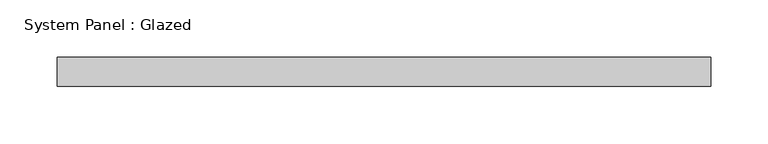
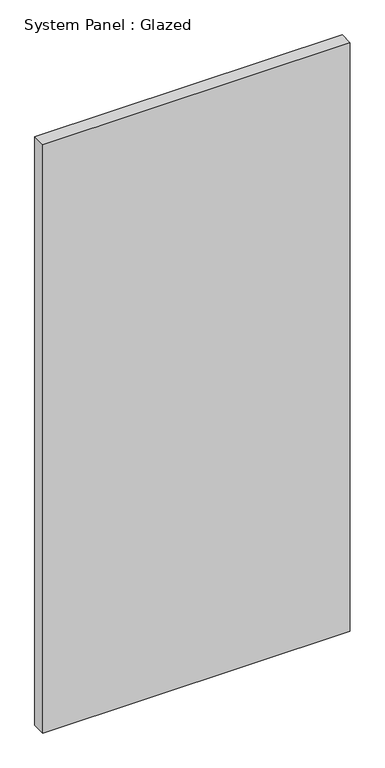
"""IFC4 building model written with IfcOpenShell, lengths in millimetres: plate geometry, System Panel : Glazed."""

from ifc_helpers import new_model, si_unit, origin, origin_with_axes, place, context, project, spatial, polyline, outline, extrude, source, transform, mapped, element, save


def system_panel_glazed_c28eec11(model_context):
    return source(origin(), model_context, "Body", "SweptSolid", [
        extrude(outline(polyline([(285.75, 19.05), (-285.75, 19.05), (-285.75, 44.45), (285.75, 44.45), (285.75, 19.05)])), origin_with_axes(), (0.0, 0.0, 1.0), 1155.7),
    ])


if __name__ == "__main__":
    model = new_model("IFC4")
    model_context = context("Model", 3, world=origin())
    ifc_project = project(units=[si_unit("LENGTHUNIT", "METRE", prefix="MILLI")], contexts=[model_context])
    site = spatial("IfcSite", under=ifc_project)
    building = spatial("IfcBuilding", under=site)
    placement = place(None, origin())
    system_panel_glazed_shape = system_panel_glazed_c28eec11(model_context)
    element("IfcPlate", 1, ObjectType="System Panel : Glazed", at=placement, inside=building, context=model_context, shape_type="MappedRepresentation", body=[
        mapped(system_panel_glazed_shape, transform((0.0, 0.0, 0.0), x_axis=(1.0, 0.0, 0.0), y_axis=(0.0, 1.0, 0.0), z_axis=(0.0, 0.0, 1.0))),
    ])
    save(model, "model.ifc")

# Revit data of these elements
# Type "System Panel : Glazed"
#   Construction Type Id = "GSP4R"
#   Analytic Construction = "1/8 in Pilkington single glazing"
#   Visual Light Transmittance = 0.9
#   Solar Heat Gain Coefficient = 0.86
#   Heat Transfer Coefficient (U) = 1.18115 BTU/(h·ft²·°F)
# Element 1 (IfcPlate, "System Panel : Glazed")
#   Materials on its faces: "Glass"
# Materials
#   "Glass": class "Glass", colour RGB 0 128 192, transparency 0.75, Description = "Soda Lime Glass", Cost = 0
